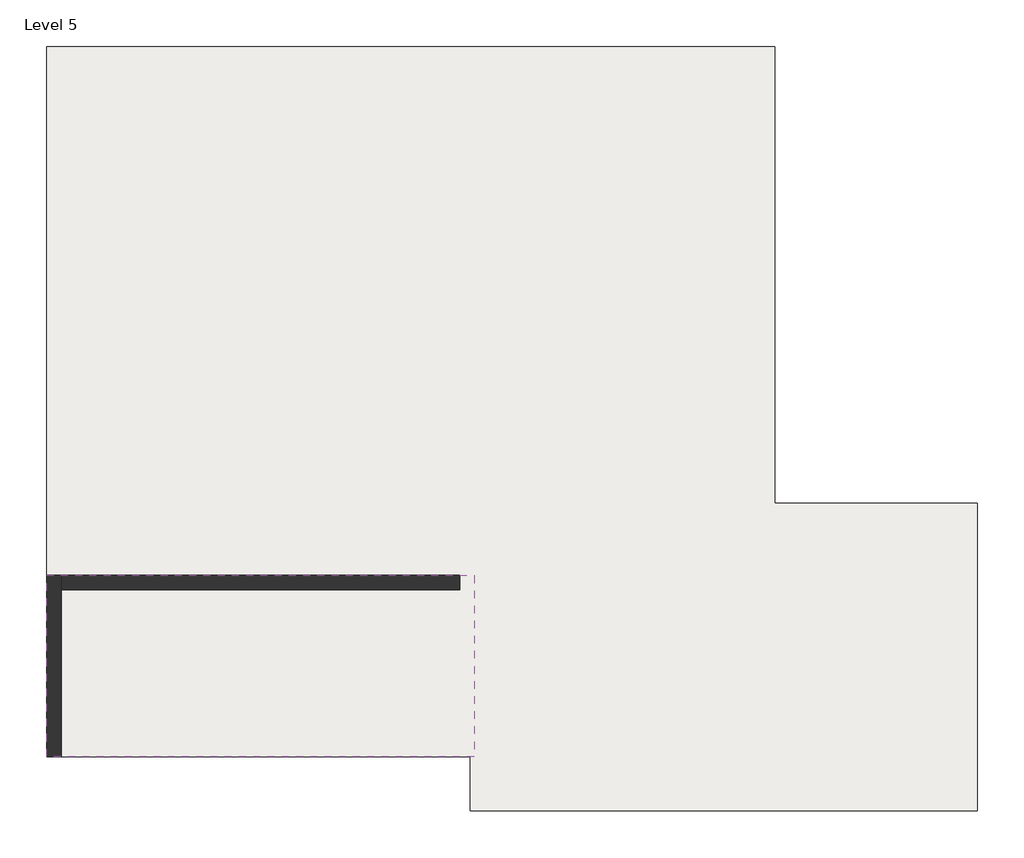
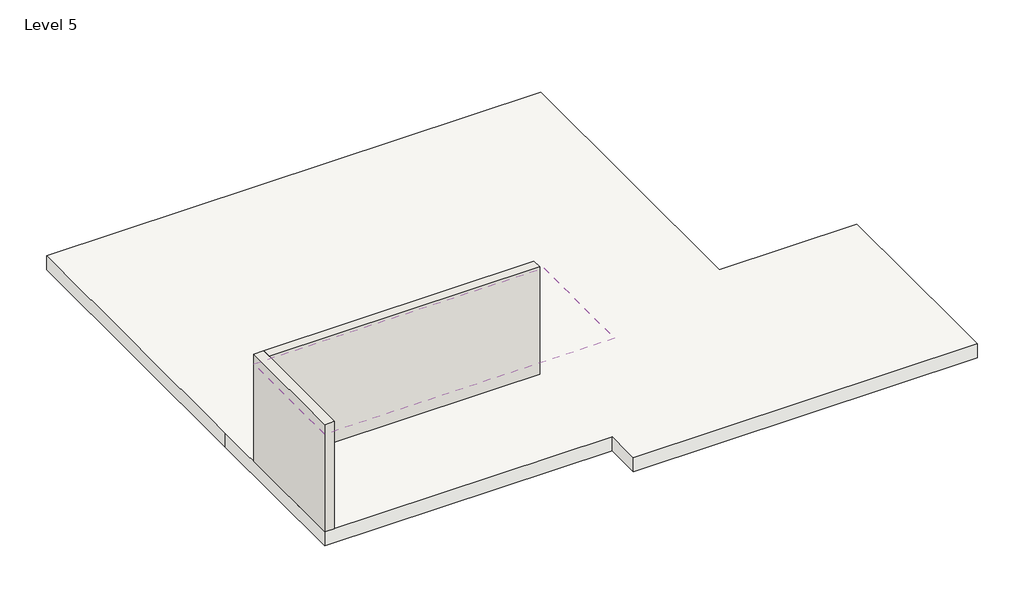
# One storey: 2 roofs, 2 walls.
"""IFC4 building model written with IfcOpenShell, lengths in millimetres."""

from ifc_helpers import new_model, si_unit, frame, origin, place, context, project, spatial, polyline, outline, extrude, faceted_brep, element, save

model = new_model("IFC4")

# Units and contexts
model_context = context("Model", 3, world=origin())
ifc_project = project(units=[si_unit("LENGTHUNIT", "METRE", prefix="MILLI")], contexts=[model_context])

# Site, building, storey
site = spatial("IfcSite", under=ifc_project)
building = spatial("IfcBuilding", under=site)
storey = spatial("IfcBuildingStorey", under=building, Name="Level 5", Elevation=14630.4)

# Roofs
placement = place(None, origin())
element("IfcRoof", 1, ObjectType="Generic - 12\"", at=placement, inside=storey, context=model_context, shape_type="SweptSolid", body=[
    extrude(outline(polyline([(-10951.9371298, 1144.5359817), (-10951.9371298, 4700.5359817), (-10951.9371298, 11101.3359817), (-741.1371298, 11101.3359817), (-741.1371298, 4700.5359817), (2101.2415497, 4700.5359817), (2101.2415497, 1144.5359817), (2101.2415497, 382.5359817), (-5008.3371298, 382.5359817), (-5008.3371298, 1144.5359817), (-10951.9371298, 1144.5359817)])), frame((0.0, 0.0, 14630.4), z_axis=(0.0, 0.0, 1.0), x_axis=(1.0, 0.0, 0.0)), (0.0, 0.0, 1.0), 304.8),
])
element("IfcRoof", 2, ObjectType="Generic - 12\"", at=placement, inside=storey, context=model_context, shape_type="SweptSolid", body=[
    extrude(outline(polyline([(-10951.9371298, 3684.5359817), (-4957.5371298, 3684.5359817), (-4957.5371298, 1144.5359817), (-10951.9371298, 1144.5359817), (-10951.9371298, 3684.5359817)])), frame((0.0, 0.0, 17068.8), z_axis=(0.0, 0.0, 1.0), x_axis=(1.0, 0.0, 0.0)), (0.0, 0.0, 1.0), 304.8),
])

# Walls
element("IfcWall", 3, ObjectType="Generic - 8\"", at=placement, inside=storey, context=model_context, shape_type="Brep", body=[
    faceted_brep([(-10748.7371298, 1144.5359817, 14935.2), (-10748.7371298, 3684.5359817, 14935.2), (-10748.7371298, 3684.5359817, 17282.1203125), (-10748.7371298, 3481.3359817, 17282.1203125), (-10748.7371298, 1144.5359817, 17282.1203125), (-10951.9371298, 1144.5359817, 14935.2), (-10951.9371298, 1144.5359817, 17282.1203125), (-10951.9371298, 3684.5359817, 17282.1203125), (-10951.9371298, 3684.5359817, 14935.2)], [[[0, 1, 2, 3, 4]], [[5, 6, 7, 8]], [[1, 0, 5, 8]], [[4, 3, 2, 7, 6]], [[2, 1, 8, 7]], [[0, 4, 6, 5]]]),
])
element("IfcWall", 4, ObjectType="Generic - 8\"", at=placement, inside=storey, context=model_context, shape_type="Brep", body=[
    faceted_brep([(-10748.7371298, 3481.3359817, 14630.4), (-5160.7371298, 3481.3359817, 14630.4), (-5160.7371298, 3481.3359817, 17282.1203125), (-10748.7371298, 3481.3359817, 17282.1203125), (-10748.7371298, 3684.5359817, 14630.4), (-10748.7371298, 3684.5359817, 14935.2), (-10748.7371298, 3684.5359817, 17282.1203125), (-5160.7371298, 3684.5359817, 17282.1203125), (-5160.7371298, 3684.5359817, 14630.4)], [[[0, 1, 2, 3]], [[4, 5, 6, 7, 8]], [[1, 0, 4, 8]], [[3, 2, 7, 6]], [[0, 3, 6, 5, 4]], [[2, 1, 8, 7]]]),
])

save(model, "model.ifc")

# Revit data of these elements
# Type "Generic - 12\""
#   Assembly Code = "B1020"
#   Layers, outside or top first: 1' - 0" no material (function 1)
# Type "Generic - 8\""
#   Assembly Code = "B2010"
#   Layers, outside or top first: 0' - 8" no material (function 1)
# Element 1 (IfcRoof, "Generic - 12\"")
#   built-in parameter 1001705 = 49 (stored number, unit not read)
#   built-in parameter 1001710 = 33615
#   Phase Created = New Construction
#   Materials on its faces: "Default Roof"
# Element 2 (IfcRoof, "Generic - 12\"")
#   built-in parameter 1001705 = 57 (stored number, unit not read)
#   built-in parameter 1001701 = 8 (stored number, unit not read)
#   built-in parameter 1001710 = 33615
#   Phase Created = New Construction
#   Materials on its faces: "Default Roof"
# Element 3 (IfcWall, "Generic - 8\"")
#   built-in parameter 1001111 = 1' - 0"
#   Top Offset = 0' - 0"
#   Base Offset = 1' - 0"
#   Unconnected Height = 7' - 8 51/128"
#   wall height = 7' - 8 51/128"
#   Phase Created = New Construction
#   Base Constraint = Level 5
#   Materials on its faces: "Default Wall"
# Element 4 (IfcWall, "Generic - 8\"")
#   Top Offset = 0' - 0"
#   Base Offset = 0' - 0"
#   Unconnected Height = 8' - 8 51/128"
#   wall height = 8' - 8 51/128"
#   Phase Created = New Construction
#   Base Constraint = Level 5
#   Materials on its faces: "Default Wall"
# Materials
#   "Default Roof": colour RGB 88 101 114, transparency 0
#   "Default Wall": colour RGB 128 128 128, transparency 0
